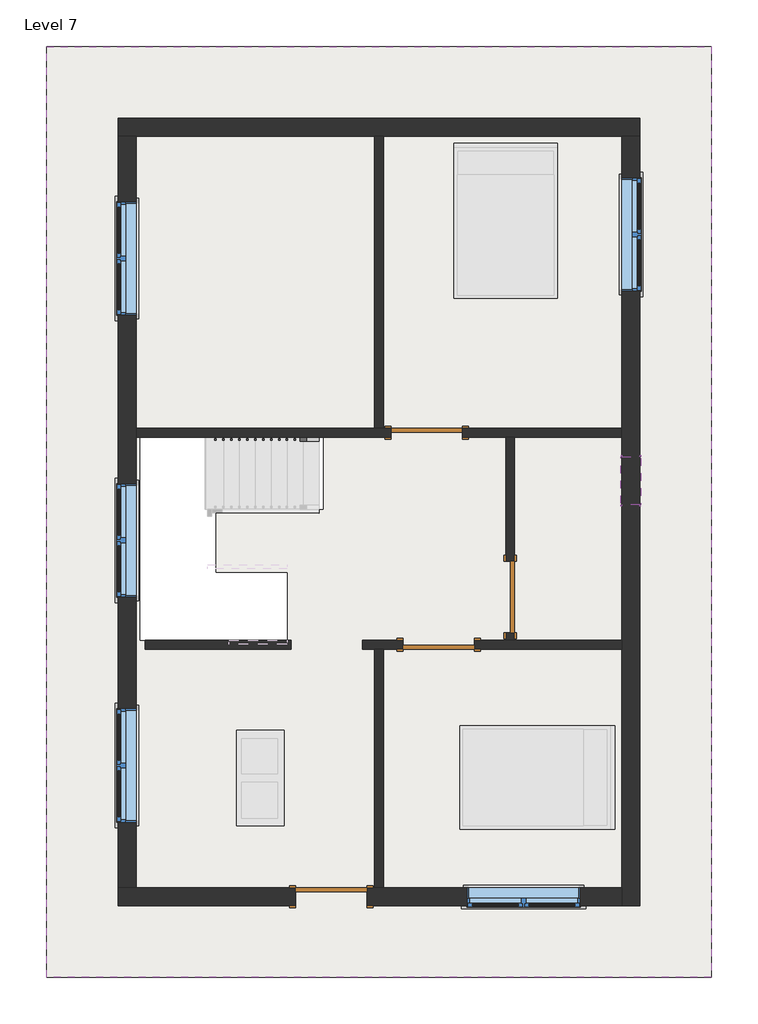
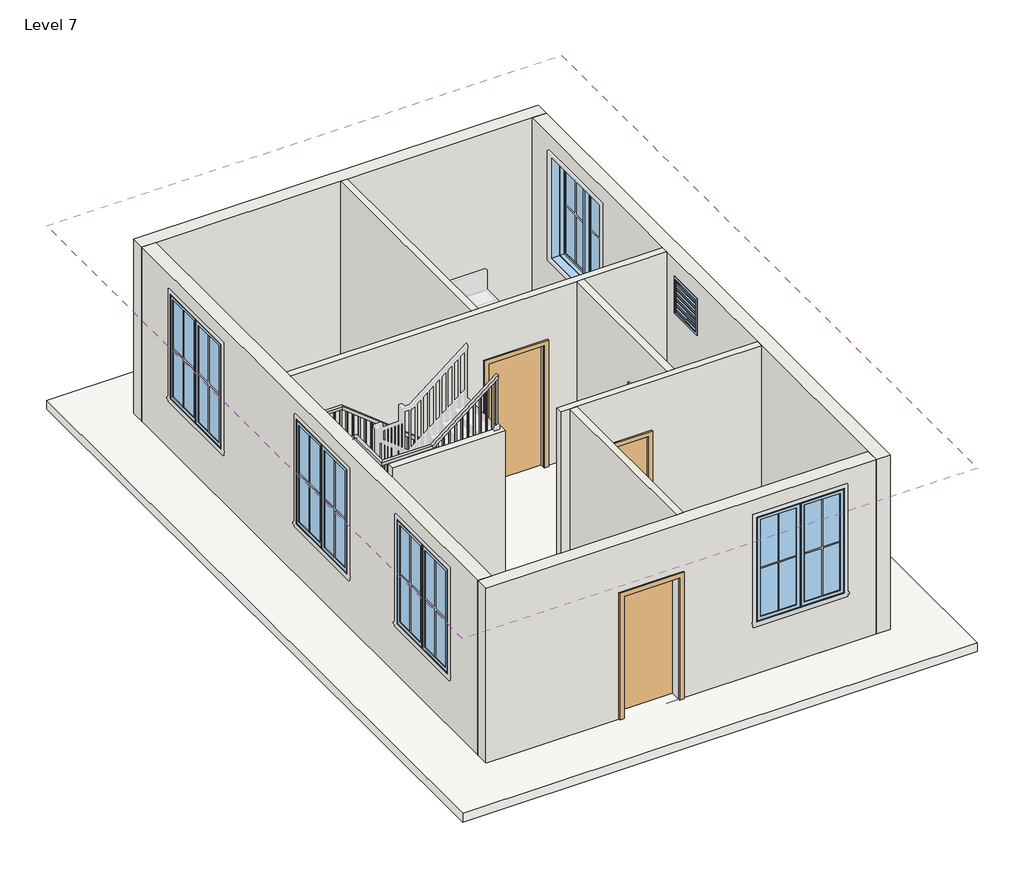
# One storey, part 1 of 2: 10 walls, 6 windows, 4 doors, 2 roofs, 1 railing, 1 slab.
"""IFC4 building model written with IfcOpenShell, lengths in millimetres."""

from ifc_helpers import new_model, si_unit, frame, origin, place, context, project, spatial, polyline, outline, extrude, faceted_brep, transform, mapped, element, save
from components import door_e5f9f3c4, door_0ca8825f, window_9ac97e1a, window_f2d8fef0

model = new_model("IFC4")

# Units and contexts
model_context = context("Model", 3, world=origin())
ifc_project = project(units=[si_unit("LENGTHUNIT", "METRE", prefix="MILLI")], contexts=[model_context])

# Site, building, storey
site = spatial("IfcSite", under=ifc_project)
building = spatial("IfcBuilding", under=site)
storey = spatial("IfcBuildingStorey", under=building, Name="Level 7", Elevation=16002.0)

# Doors
placement = place(None, origin())
door_shape = door_e5f9f3c4(model_context)
element("IfcDoor", 1, ObjectType="Single-Flush : 36\" x 84\"", at=placement, inside=storey, context=model_context, shape_type="MappedRepresentation", body=[
    mapped(door_shape, transform((-2225.1840247, 979.1819954, 16002.0), x_axis=(1.0, 0.0, 0.0), y_axis=(0.0, 1.0, 0.0), z_axis=(0.0, 0.0, 1.0))),
])
element("IfcDoor", 2, ObjectType="Single-Flush : 36\" x 84\"", at=placement, inside=storey, context=model_context, shape_type="MappedRepresentation", body=[
    mapped(door_shape, transform((-1158.3840247, -1116.3180046, 16002.0), x_axis=(0.0, -1.0, 0.0), y_axis=(1.0, 0.0, 0.0), z_axis=(0.0, 0.0, 1.0))),
])
element("IfcDoor", 3, ObjectType="Single-Flush : 36\" x 84\"", at=placement, inside=storey, context=model_context, shape_type="MappedRepresentation", body=[
    mapped(door_shape, transform((-2072.7840247, -1725.9180046, 16002.0), x_axis=(-1.0, 0.0, 0.0), y_axis=(0.0, -1.0, 0.0), z_axis=(0.0, 0.0, 1.0))),
])
door_2_shape = door_0ca8825f(model_context)
element("IfcDoor", 4, ObjectType="Single-Flush : 36\" x 84\"", at=placement, inside=storey, context=model_context, shape_type="MappedRepresentation", body=[
    mapped(door_2_shape, transform((-3444.3840247, -4945.3680046, 16002.0), x_axis=(1.0, 0.0, 0.0), y_axis=(0.0, 1.0, 0.0), z_axis=(0.0, 0.0, 1.0))),
])

# Railing
element("IfcRailing", 5, ObjectType="Handrail - Rectangular", at=placement, inside=storey, context=model_context, shape_type="SolidModel", body=[
    faceted_brep([(-3603.1340247, 871.2319954, 17076.8210526), (-3603.1340247, 871.2319954, 17012.0980109), (-3603.1340247, 922.0319954, 17012.0980109), (-3603.1340247, 922.0319954, 17076.8210526), (-5097.5006913, 871.2319954, 18256.5842105), (-5115.1365442, 871.2319954, 18205.7842105), (-5115.1365442, 922.0319954, 18205.7842105), (-5097.5006913, 922.0319954, 18256.5842105), (-5889.1340247, 871.2319954, 18256.5842105), (-5889.1340247, 871.2319954, 18205.7842105), (-5939.9340247, 922.0319954, 18205.7842105), (-5939.9340247, 922.0319954, 18256.5842105), (-5889.1340247, 130.6632454, 18256.5842105), (-5889.1340247, 112.1228815, 18205.7842105), (-5939.9340247, 112.1228815, 18205.7842105), (-5939.9340247, 130.6632454, 18256.5842105), (-5889.1340247, -877.3992546, 19105.4789474), (-5889.1340247, -895.9396185, 19054.6789474), (-5939.9340247, -895.9396185, 19054.6789474), (-5939.9340247, -877.3992546, 19105.4789474), (-5889.1340247, -1617.9680046, 19105.4789474), (-5889.1340247, -1617.9680046, 19054.6789474), (-5939.9340247, -1668.7680046, 19054.6789474), (-5939.9340247, -1668.7680046, 19105.4789474), (-5097.5006913, -1617.9680046, 19105.4789474), (-5079.8648385, -1617.9680046, 19054.6789474), (-5079.8648385, -1668.7680046, 19054.6789474), (-5097.5006913, -1668.7680046, 19105.4789474), (-4009.5340247, -1617.9680046, 19964.4), (-4009.5340247, -1668.7680046, 19964.4), (-4009.5340247, -1668.7680046, 19899.6769583), (-4009.5340247, -1617.9680046, 19899.6769583)], [[[0, 1, 2, 3]], [[1, 0, 4, 5]], [[2, 1, 5, 6]], [[3, 2, 6, 7]], [[0, 3, 7, 4]], [[5, 4, 8, 9]], [[6, 5, 9, 10]], [[7, 6, 10, 11]], [[4, 7, 11, 8]], [[9, 8, 12, 13]], [[10, 9, 13, 14]], [[11, 10, 14, 15]], [[8, 11, 15, 12]], [[13, 12, 16, 17]], [[14, 13, 17, 18]], [[15, 14, 18, 19]], [[12, 15, 19, 16]], [[17, 16, 20, 21]], [[18, 17, 21, 22]], [[19, 18, 22, 23]], [[16, 19, 23, 20]], [[21, 20, 24, 25]], [[22, 21, 25, 26]], [[23, 22, 26, 27]], [[20, 23, 27, 24]], [[28, 29, 30, 31]], [[25, 24, 28, 31]], [[26, 25, 31, 30]], [[27, 26, 30, 29]], [[24, 27, 29, 28]]]),
    extrude(outline(polyline([(19847.0388004, -4076.2090247), (19831.9993267, -4095.2590247), (18889.5789474, -4095.2590247), (18889.5789474, -4076.2090247), (19847.0388004, -4076.2090247)])), frame((0.0, -1652.8930046, 0.0), z_axis=(0.0, 1.0, 0.0), x_axis=(0.0, 0.0, 1.0)), (0.0, 0.0, 1.0), 19.05),
    extrude(outline(polyline([(19766.828274, -4177.8090247), (19751.7888004, -4196.8590247), (18889.5789474, -4196.8590247), (18889.5789474, -4177.8090247), (19766.828274, -4177.8090247)])), frame((0.0, -1652.8930046, 0.0), z_axis=(0.0, 1.0, 0.0), x_axis=(0.0, 0.0, 1.0)), (0.0, 0.0, 1.0), 19.05),
    extrude(outline(polyline([(19686.6177477, -4279.4090247), (19671.578274, -4298.4590247), (18729.1578947, -4298.4590247), (18729.1578947, -4279.4090247), (19686.6177477, -4279.4090247)])), frame((0.0, -1652.8930046, 0.0), z_axis=(0.0, 1.0, 0.0), x_axis=(0.0, 0.0, 1.0)), (0.0, 0.0, 1.0), 19.05),
    extrude(outline(polyline([(19606.4072214, -4381.0090247), (19591.3677477, -4400.0590247), (18729.1578947, -4400.0590247), (18729.1578947, -4381.0090247), (19606.4072214, -4381.0090247)])), frame((0.0, -1652.8930046, 0.0), z_axis=(0.0, 1.0, 0.0), x_axis=(0.0, 0.0, 1.0)), (0.0, 0.0, 1.0), 19.05),
    extrude(outline(polyline([(19526.1966951, -4482.6090247), (19511.1572214, -4501.6590247), (18568.7368421, -4501.6590247), (18568.7368421, -4482.6090247), (19526.1966951, -4482.6090247)])), frame((0.0, -1652.8930046, 0.0), z_axis=(0.0, 1.0, 0.0), x_axis=(0.0, 0.0, 1.0)), (0.0, 0.0, 1.0), 19.05),
    extrude(outline(polyline([(19445.9861688, -4584.2090247), (19430.9466951, -4603.2590247), (18568.7368421, -4603.2590247), (18568.7368421, -4584.2090247), (19445.9861688, -4584.2090247)])), frame((0.0, -1652.8930046, 0.0), z_axis=(0.0, 1.0, 0.0), x_axis=(0.0, 0.0, 1.0)), (0.0, 0.0, 1.0), 19.05),
    extrude(outline(polyline([(19365.7756425, -4685.8090247), (19350.7361688, -4704.8590247), (18408.3157895, -4704.8590247), (18408.3157895, -4685.8090247), (19365.7756425, -4685.8090247)])), frame((0.0, -1652.8930046, 0.0), z_axis=(0.0, 1.0, 0.0), x_axis=(0.0, 0.0, 1.0)), (0.0, 0.0, 1.0), 19.05),
    extrude(outline(polyline([(19285.5651161, -4787.4090247), (19270.5256425, -4806.4590247), (18408.3157895, -4806.4590247), (18408.3157895, -4787.4090247), (19285.5651161, -4787.4090247)])), frame((0.0, -1652.8930046, 0.0), z_axis=(0.0, 1.0, 0.0), x_axis=(0.0, 0.0, 1.0)), (0.0, 0.0, 1.0), 19.05),
    extrude(outline(polyline([(19205.3545898, -4889.0090247), (19190.3151161, -4908.0590247), (18247.8947368, -4908.0590247), (18247.8947368, -4889.0090247), (19205.3545898, -4889.0090247)])), frame((0.0, -1652.8930046, 0.0), z_axis=(0.0, 1.0, 0.0), x_axis=(0.0, 0.0, 1.0)), (0.0, 0.0, 1.0), 19.05),
    extrude(outline(polyline([(19125.1440635, -4990.6090247), (19110.1045898, -5009.6590247), (18247.8947368, -5009.6590247), (18247.8947368, -4990.6090247), (19125.1440635, -4990.6090247)])), frame((0.0, -1652.8930046, 0.0), z_axis=(0.0, 1.0, 0.0), x_axis=(0.0, 0.0, 1.0)), (0.0, 0.0, 1.0), 19.05),
    extrude(outline(polyline([(-5111.2590247, -1652.8930046), (-5111.2590247, -1633.8430046), (-5092.2090247, -1633.8430046), (-5092.2090247, -1652.8930046), (-5111.2590247, -1652.8930046)])), frame((0.0, 0.0, 18087.4736842), z_axis=(0.0, 0.0, 1.0), x_axis=(1.0, 0.0, 0.0)), (0.0, 0.0, 1.0), 967.2052632),
    extrude(outline(polyline([(-5212.8590247, -1652.8930046), (-5212.8590247, -1633.8430046), (-5193.8090247, -1633.8430046), (-5193.8090247, -1652.8930046), (-5212.8590247, -1652.8930046)])), frame((0.0, 0.0, 18087.4736842), z_axis=(0.0, 0.0, 1.0), x_axis=(1.0, 0.0, 0.0)), (0.0, 0.0, 1.0), 967.2052632),
    extrude(outline(polyline([(-5314.4590247, -1652.8930046), (-5314.4590247, -1633.8430046), (-5295.4090247, -1633.8430046), (-5295.4090247, -1652.8930046), (-5314.4590247, -1652.8930046)])), frame((0.0, 0.0, 18087.4736842), z_axis=(0.0, 0.0, 1.0), x_axis=(1.0, 0.0, 0.0)), (0.0, 0.0, 1.0), 967.2052632),
    extrude(outline(polyline([(-5416.0590247, -1652.8930046), (-5416.0590247, -1633.8430046), (-5397.0090247, -1633.8430046), (-5397.0090247, -1652.8930046), (-5416.0590247, -1652.8930046)])), frame((0.0, 0.0, 18087.4736842), z_axis=(0.0, 0.0, 1.0), x_axis=(1.0, 0.0, 0.0)), (0.0, 0.0, 1.0), 967.2052632),
    extrude(outline(polyline([(-5517.6590247, -1652.8930046), (-5517.6590247, -1633.8430046), (-5498.6090247, -1633.8430046), (-5498.6090247, -1652.8930046), (-5517.6590247, -1652.8930046)])), frame((0.0, 0.0, 18087.4736842), z_axis=(0.0, 0.0, 1.0), x_axis=(1.0, 0.0, 0.0)), (0.0, 0.0, 1.0), 967.2052632),
    extrude(outline(polyline([(-5619.2590247, -1652.8930046), (-5619.2590247, -1633.8430046), (-5600.2090247, -1633.8430046), (-5600.2090247, -1652.8930046), (-5619.2590247, -1652.8930046)])), frame((0.0, 0.0, 18087.4736842), z_axis=(0.0, 0.0, 1.0), x_axis=(1.0, 0.0, 0.0)), (0.0, 0.0, 1.0), 967.2052632),
    extrude(outline(polyline([(-5720.8590247, -1652.8930046), (-5720.8590247, -1633.8430046), (-5701.8090247, -1633.8430046), (-5701.8090247, -1652.8930046), (-5720.8590247, -1652.8930046)])), frame((0.0, 0.0, 18087.4736842), z_axis=(0.0, 0.0, 1.0), x_axis=(1.0, 0.0, 0.0)), (0.0, 0.0, 1.0), 967.2052632),
    extrude(outline(polyline([(-5822.4590247, -1652.8930046), (-5822.4590247, -1633.8430046), (-5803.4090247, -1633.8430046), (-5803.4090247, -1652.8930046), (-5822.4590247, -1652.8930046)])), frame((0.0, 0.0, 18087.4736842), z_axis=(0.0, 0.0, 1.0), x_axis=(1.0, 0.0, 0.0)), (0.0, 0.0, 1.0), 967.2052632),
    extrude(outline(polyline([(-5924.0590247, -1532.2430046), (-5905.0090247, -1532.2430046), (-5905.0090247, -1551.2930046), (-5924.0590247, -1551.2930046), (-5924.0590247, -1532.2430046)])), frame((0.0, 0.0, 18087.4736842), z_axis=(0.0, 0.0, 1.0), x_axis=(1.0, 0.0, 0.0)), (0.0, 0.0, 1.0), 967.2052632),
    extrude(outline(polyline([(-5924.0590247, -1430.6430046), (-5905.0090247, -1430.6430046), (-5905.0090247, -1449.6930046), (-5924.0590247, -1449.6930046), (-5924.0590247, -1430.6430046)])), frame((0.0, 0.0, 18087.4736842), z_axis=(0.0, 0.0, 1.0), x_axis=(1.0, 0.0, 0.0)), (0.0, 0.0, 1.0), 967.2052632),
    extrude(outline(polyline([(-5924.0590247, -1329.0430046), (-5905.0090247, -1329.0430046), (-5905.0090247, -1348.0930046), (-5924.0590247, -1348.0930046), (-5924.0590247, -1329.0430046)])), frame((0.0, 0.0, 18087.4736842), z_axis=(0.0, 0.0, 1.0), x_axis=(1.0, 0.0, 0.0)), (0.0, 0.0, 1.0), 967.2052632),
    extrude(outline(polyline([(-5924.0590247, -1227.4430046), (-5905.0090247, -1227.4430046), (-5905.0090247, -1246.4930046), (-5924.0590247, -1246.4930046), (-5924.0590247, -1227.4430046)])), frame((0.0, 0.0, 18087.4736842), z_axis=(0.0, 0.0, 1.0), x_axis=(1.0, 0.0, 0.0)), (0.0, 0.0, 1.0), 967.2052632),
    extrude(outline(polyline([(-5924.0590247, -1125.8430046), (-5905.0090247, -1125.8430046), (-5905.0090247, -1144.8930046), (-5924.0590247, -1144.8930046), (-5924.0590247, -1125.8430046)])), frame((0.0, 0.0, 18087.4736842), z_axis=(0.0, 0.0, 1.0), x_axis=(1.0, 0.0, 0.0)), (0.0, 0.0, 1.0), 967.2052632),
    extrude(outline(polyline([(-5924.0590247, -1024.2430046), (-5905.0090247, -1024.2430046), (-5905.0090247, -1043.2930046), (-5924.0590247, -1043.2930046), (-5924.0590247, -1024.2430046)])), frame((0.0, 0.0, 18087.4736842), z_axis=(0.0, 0.0, 1.0), x_axis=(1.0, 0.0, 0.0)), (0.0, 0.0, 1.0), 967.2052632),
    extrude(outline(polyline([(-5924.0590247, -922.6430046), (-5905.0090247, -922.6430046), (-5905.0090247, -941.6930046), (-5924.0590247, -941.6930046), (-5924.0590247, -922.6430046)])), frame((0.0, 0.0, 18087.4736842), z_axis=(0.0, 0.0, 1.0), x_axis=(1.0, 0.0, 0.0)), (0.0, 0.0, 1.0), 967.2052632),
    extrude(outline(polyline([(-840.0930046, 19007.6502199), (-821.0430046, 18991.6081146), (-821.0430046, 18087.4736842), (-840.0930046, 18087.4736842), (-840.0930046, 19007.6502199)])), frame((-5924.0590247, 0.0, 0.0), z_axis=(1.0, 0.0, 0.0), x_axis=(0.0, 1.0, 0.0)), (0.0, 0.0, 1.0), 19.05),
    extrude(outline(polyline([(-738.4930046, 18922.0923251), (-719.4430046, 18906.0502199), (-719.4430046, 17927.0526316), (-738.4930046, 17927.0526316), (-738.4930046, 18922.0923251)])), frame((-5924.0590247, 0.0, 0.0), z_axis=(1.0, 0.0, 0.0), x_axis=(0.0, 1.0, 0.0)), (0.0, 0.0, 1.0), 19.05),
    extrude(outline(polyline([(-636.8930046, 18836.5344304), (-617.8430046, 18820.4923251), (-617.8430046, 17927.0526316), (-636.8930046, 17927.0526316), (-636.8930046, 18836.5344304)])), frame((-5924.0590247, 0.0, 0.0), z_axis=(1.0, 0.0, 0.0), x_axis=(0.0, 1.0, 0.0)), (0.0, 0.0, 1.0), 19.05),
    extrude(outline(polyline([(-535.2930046, 18750.9765357), (-516.2430046, 18734.9344304), (-516.2430046, 17766.6315789), (-535.2930046, 17766.6315789), (-535.2930046, 18750.9765357)])), frame((-5924.0590247, 0.0, 0.0), z_axis=(1.0, 0.0, 0.0), x_axis=(0.0, 1.0, 0.0)), (0.0, 0.0, 1.0), 19.05),
    extrude(outline(polyline([(-433.6930046, 18665.4186409), (-414.6430046, 18649.3765357), (-414.6430046, 17766.6315789), (-433.6930046, 17766.6315789), (-433.6930046, 18665.4186409)])), frame((-5924.0590247, 0.0, 0.0), z_axis=(1.0, 0.0, 0.0), x_axis=(0.0, 1.0, 0.0)), (0.0, 0.0, 1.0), 19.05),
    extrude(outline(polyline([(-332.0930046, 18579.8607462), (-313.0430046, 18563.8186409), (-313.0430046, 17606.2105263), (-332.0930046, 17606.2105263), (-332.0930046, 18579.8607462)])), frame((-5924.0590247, 0.0, 0.0), z_axis=(1.0, 0.0, 0.0), x_axis=(0.0, 1.0, 0.0)), (0.0, 0.0, 1.0), 19.05),
    extrude(outline(polyline([(-230.4930046, 18494.3028514), (-211.4430046, 18478.2607462), (-211.4430046, 17606.2105263), (-230.4930046, 17606.2105263), (-230.4930046, 18494.3028514)])), frame((-5924.0590247, 0.0, 0.0), z_axis=(1.0, 0.0, 0.0), x_axis=(0.0, 1.0, 0.0)), (0.0, 0.0, 1.0), 19.05),
    extrude(outline(polyline([(-128.8930046, 18408.7449567), (-109.8430046, 18392.7028514), (-109.8430046, 17445.7894737), (-128.8930046, 17445.7894737), (-128.8930046, 18408.7449567)])), frame((-5924.0590247, 0.0, 0.0), z_axis=(1.0, 0.0, 0.0), x_axis=(0.0, 1.0, 0.0)), (0.0, 0.0, 1.0), 19.05),
    extrude(outline(polyline([(-27.2930046, 18323.187062), (-8.2430046, 18307.1449567), (-8.2430046, 17445.7894737), (-27.2930046, 17445.7894737), (-27.2930046, 18323.187062)])), frame((-5924.0590247, 0.0, 0.0), z_axis=(1.0, 0.0, 0.0), x_axis=(0.0, 1.0, 0.0)), (0.0, 0.0, 1.0), 19.05),
    extrude(outline(polyline([(74.3069954, 18237.6291672), (93.3569954, 18221.587062), (93.3569954, 17285.3684211), (74.3069954, 17285.3684211), (74.3069954, 18237.6291672)])), frame((-5924.0590247, 0.0, 0.0), z_axis=(1.0, 0.0, 0.0), x_axis=(0.0, 1.0, 0.0)), (0.0, 0.0, 1.0), 19.05),
    extrude(outline(polyline([(-5924.0590247, 194.9569954), (-5905.0090247, 194.9569954), (-5905.0090247, 175.9069954), (-5924.0590247, 175.9069954), (-5924.0590247, 194.9569954)])), frame((0.0, 0.0, 17285.3684211), z_axis=(0.0, 0.0, 1.0), x_axis=(1.0, 0.0, 0.0)), (0.0, 0.0, 1.0), 920.4157895),
    extrude(outline(polyline([(-5924.0590247, 296.5569954), (-5905.0090247, 296.5569954), (-5905.0090247, 277.5069954), (-5924.0590247, 277.5069954), (-5924.0590247, 296.5569954)])), frame((0.0, 0.0, 17285.3684211), z_axis=(0.0, 0.0, 1.0), x_axis=(1.0, 0.0, 0.0)), (0.0, 0.0, 1.0), 920.4157895),
    extrude(outline(polyline([(-5924.0590247, 398.1569954), (-5905.0090247, 398.1569954), (-5905.0090247, 379.1069954), (-5924.0590247, 379.1069954), (-5924.0590247, 398.1569954)])), frame((0.0, 0.0, 17285.3684211), z_axis=(0.0, 0.0, 1.0), x_axis=(1.0, 0.0, 0.0)), (0.0, 0.0, 1.0), 920.4157895),
    extrude(outline(polyline([(-5924.0590247, 499.7569954), (-5905.0090247, 499.7569954), (-5905.0090247, 480.7069954), (-5924.0590247, 480.7069954), (-5924.0590247, 499.7569954)])), frame((0.0, 0.0, 17285.3684211), z_axis=(0.0, 0.0, 1.0), x_axis=(1.0, 0.0, 0.0)), (0.0, 0.0, 1.0), 920.4157895),
    extrude(outline(polyline([(-5924.0590247, 601.3569954), (-5905.0090247, 601.3569954), (-5905.0090247, 582.3069954), (-5924.0590247, 582.3069954), (-5924.0590247, 601.3569954)])), frame((0.0, 0.0, 17285.3684211), z_axis=(0.0, 0.0, 1.0), x_axis=(1.0, 0.0, 0.0)), (0.0, 0.0, 1.0), 920.4157895),
    extrude(outline(polyline([(-5924.0590247, 702.9569954), (-5905.0090247, 702.9569954), (-5905.0090247, 683.9069954), (-5924.0590247, 683.9069954), (-5924.0590247, 702.9569954)])), frame((0.0, 0.0, 17285.3684211), z_axis=(0.0, 0.0, 1.0), x_axis=(1.0, 0.0, 0.0)), (0.0, 0.0, 1.0), 920.4157895),
    extrude(outline(polyline([(-5924.0590247, 804.5569954), (-5905.0090247, 804.5569954), (-5905.0090247, 785.5069954), (-5924.0590247, 785.5069954), (-5924.0590247, 804.5569954)])), frame((0.0, 0.0, 17285.3684211), z_axis=(0.0, 0.0, 1.0), x_axis=(1.0, 0.0, 0.0)), (0.0, 0.0, 1.0), 920.4157895),
    extrude(outline(polyline([(-5828.8090247, 906.1569954), (-5828.8090247, 887.1069954), (-5847.8590247, 887.1069954), (-5847.8590247, 906.1569954), (-5828.8090247, 906.1569954)])), frame((0.0, 0.0, 17285.3684211), z_axis=(0.0, 0.0, 1.0), x_axis=(1.0, 0.0, 0.0)), (0.0, 0.0, 1.0), 920.4157895),
    extrude(outline(polyline([(-5727.2090247, 906.1569954), (-5727.2090247, 887.1069954), (-5746.2590247, 887.1069954), (-5746.2590247, 906.1569954), (-5727.2090247, 906.1569954)])), frame((0.0, 0.0, 17285.3684211), z_axis=(0.0, 0.0, 1.0), x_axis=(1.0, 0.0, 0.0)), (0.0, 0.0, 1.0), 920.4157895),
    extrude(outline(polyline([(-5625.6090247, 906.1569954), (-5625.6090247, 887.1069954), (-5644.6590247, 887.1069954), (-5644.6590247, 906.1569954), (-5625.6090247, 906.1569954)])), frame((0.0, 0.0, 17285.3684211), z_axis=(0.0, 0.0, 1.0), x_axis=(1.0, 0.0, 0.0)), (0.0, 0.0, 1.0), 920.4157895),
    extrude(outline(polyline([(-5524.0090247, 906.1569954), (-5524.0090247, 887.1069954), (-5543.0590247, 887.1069954), (-5543.0590247, 906.1569954), (-5524.0090247, 906.1569954)])), frame((0.0, 0.0, 17285.3684211), z_axis=(0.0, 0.0, 1.0), x_axis=(1.0, 0.0, 0.0)), (0.0, 0.0, 1.0), 920.4157895),
    extrude(outline(polyline([(-5422.4090247, 906.1569954), (-5422.4090247, 887.1069954), (-5441.4590247, 887.1069954), (-5441.4590247, 906.1569954), (-5422.4090247, 906.1569954)])), frame((0.0, 0.0, 17285.3684211), z_axis=(0.0, 0.0, 1.0), x_axis=(1.0, 0.0, 0.0)), (0.0, 0.0, 1.0), 920.4157895),
    extrude(outline(polyline([(-5320.8090247, 906.1569954), (-5320.8090247, 887.1069954), (-5339.8590247, 887.1069954), (-5339.8590247, 906.1569954), (-5320.8090247, 906.1569954)])), frame((0.0, 0.0, 17285.3684211), z_axis=(0.0, 0.0, 1.0), x_axis=(1.0, 0.0, 0.0)), (0.0, 0.0, 1.0), 920.4157895),
    extrude(outline(polyline([(-5219.2090247, 906.1569954), (-5219.2090247, 887.1069954), (-5238.2590247, 887.1069954), (-5238.2590247, 906.1569954), (-5219.2090247, 906.1569954)])), frame((0.0, 0.0, 17285.3684211), z_axis=(0.0, 0.0, 1.0), x_axis=(1.0, 0.0, 0.0)), (0.0, 0.0, 1.0), 920.4157895),
    extrude(outline(polyline([(-5117.6090247, 906.1569954), (-5117.6090247, 887.1069954), (-5136.6590247, 887.1069954), (-5136.6590247, 906.1569954), (-5117.6090247, 906.1569954)])), frame((0.0, 0.0, 17285.3684211), z_axis=(0.0, 0.0, 1.0), x_axis=(1.0, 0.0, 0.0)), (0.0, 0.0, 1.0), 920.4157895),
    extrude(outline(polyline([(18127.5256425, -5016.0090247), (18142.5651161, -5035.0590247), (17285.3684211, -5035.0590247), (17285.3684211, -5016.0090247), (18127.5256425, -5016.0090247)])), frame((0.0, 887.1069954, 0.0), z_axis=(0.0, 1.0, 0.0), x_axis=(0.0, 0.0, 1.0)), (0.0, 0.0, 1.0), 19.05),
    extrude(outline(polyline([(18047.3151161, -4914.4090247), (18062.3545898, -4933.4590247), (17124.9473684, -4933.4590247), (17124.9473684, -4914.4090247), (18047.3151161, -4914.4090247)])), frame((0.0, 887.1069954, 0.0), z_axis=(0.0, 1.0, 0.0), x_axis=(0.0, 0.0, 1.0)), (0.0, 0.0, 1.0), 19.05),
    extrude(outline(polyline([(17967.1045898, -4812.8090247), (17982.1440635, -4831.8590247), (17124.9473684, -4831.8590247), (17124.9473684, -4812.8090247), (17967.1045898, -4812.8090247)])), frame((0.0, 887.1069954, 0.0), z_axis=(0.0, 1.0, 0.0), x_axis=(0.0, 0.0, 1.0)), (0.0, 0.0, 1.0), 19.05),
    extrude(outline(polyline([(17886.8940635, -4711.2090247), (17901.9335372, -4730.2590247), (16964.5263158, -4730.2590247), (16964.5263158, -4711.2090247), (17886.8940635, -4711.2090247)])), frame((0.0, 887.1069954, 0.0), z_axis=(0.0, 1.0, 0.0), x_axis=(0.0, 0.0, 1.0)), (0.0, 0.0, 1.0), 19.05),
    extrude(outline(polyline([(17806.6835372, -4609.6090247), (17821.7230109, -4628.6590247), (16964.5263158, -4628.6590247), (16964.5263158, -4609.6090247), (17806.6835372, -4609.6090247)])), frame((0.0, 887.1069954, 0.0), z_axis=(0.0, 1.0, 0.0), x_axis=(0.0, 0.0, 1.0)), (0.0, 0.0, 1.0), 19.05),
    extrude(outline(polyline([(17726.4730109, -4508.0090247), (17741.5124846, -4527.0590247), (16804.1052632, -4527.0590247), (16804.1052632, -4508.0090247), (17726.4730109, -4508.0090247)])), frame((0.0, 887.1069954, 0.0), z_axis=(0.0, 1.0, 0.0), x_axis=(0.0, 0.0, 1.0)), (0.0, 0.0, 1.0), 19.05),
    extrude(outline(polyline([(17646.2624846, -4406.4090247), (17661.3019583, -4425.4590247), (16804.1052632, -4425.4590247), (16804.1052632, -4406.4090247), (17646.2624846, -4406.4090247)])), frame((0.0, 887.1069954, 0.0), z_axis=(0.0, 1.0, 0.0), x_axis=(0.0, 0.0, 1.0)), (0.0, 0.0, 1.0), 19.05),
    extrude(outline(polyline([(17566.0519583, -4304.8090247), (17581.0914319, -4323.8590247), (16643.6842105, -4323.8590247), (16643.6842105, -4304.8090247), (17566.0519583, -4304.8090247)])), frame((0.0, 887.1069954, 0.0), z_axis=(0.0, 1.0, 0.0), x_axis=(0.0, 0.0, 1.0)), (0.0, 0.0, 1.0), 19.05),
    extrude(outline(polyline([(17485.8414319, -4203.2090247), (17500.8809056, -4222.2590247), (16643.6842105, -4222.2590247), (16643.6842105, -4203.2090247), (17485.8414319, -4203.2090247)])), frame((0.0, 887.1069954, 0.0), z_axis=(0.0, 1.0, 0.0), x_axis=(0.0, 0.0, 1.0)), (0.0, 0.0, 1.0), 19.05),
    extrude(outline(polyline([(17405.6309056, -4101.6090247), (17420.6703793, -4120.6590247), (16483.2631579, -4120.6590247), (16483.2631579, -4101.6090247), (17405.6309056, -4101.6090247)])), frame((0.0, 887.1069954, 0.0), z_axis=(0.0, 1.0, 0.0), x_axis=(0.0, 0.0, 1.0)), (0.0, 0.0, 1.0), 19.05),
    extrude(outline(polyline([(17325.4203793, -4000.0090247), (17340.459853, -4019.0590247), (16483.2631579, -4019.0590247), (16483.2631579, -4000.0090247), (17325.4203793, -4000.0090247)])), frame((0.0, 887.1069954, 0.0), z_axis=(0.0, 1.0, 0.0), x_axis=(0.0, 0.0, 1.0)), (0.0, 0.0, 1.0), 19.05),
    extrude(outline(polyline([(17245.209853, -3898.4090247), (17260.2493267, -3917.4590247), (16322.8421053, -3917.4590247), (16322.8421053, -3898.4090247), (17245.209853, -3898.4090247)])), frame((0.0, 887.1069954, 0.0), z_axis=(0.0, 1.0, 0.0), x_axis=(0.0, 0.0, 1.0)), (0.0, 0.0, 1.0), 19.05),
    extrude(outline(polyline([(17164.9993267, -3796.8090247), (17180.0388004, -3815.8590247), (16322.8421053, -3815.8590247), (16322.8421053, -3796.8090247), (17164.9993267, -3796.8090247)])), frame((0.0, 887.1069954, 0.0), z_axis=(0.0, 1.0, 0.0), x_axis=(0.0, 0.0, 1.0)), (0.0, 0.0, 1.0), 19.05),
    extrude(outline(polyline([(17084.7888004, -3695.2090247), (17099.828274, -3714.2590247), (16162.4210526, -3714.2590247), (16162.4210526, -3695.2090247), (17084.7888004, -3695.2090247)])), frame((0.0, 887.1069954, 0.0), z_axis=(0.0, 1.0, 0.0), x_axis=(0.0, 0.0, 1.0)), (0.0, 0.0, 1.0), 19.05),
    extrude(outline(polyline([(-5924.0590247, -1633.8430046), (-5905.0090247, -1633.8430046), (-5905.0090247, -1652.8930046), (-5924.0590247, -1652.8930046), (-5924.0590247, -1633.8430046)])), frame((0.0, 0.0, 18087.4736842), z_axis=(0.0, 0.0, 1.0), x_axis=(1.0, 0.0, 0.0)), (0.0, 0.0, 1.0), 967.2052632),
    extrude(outline(polyline([(-5905.0090247, 906.1569954), (-5905.0090247, 887.1069954), (-5924.0590247, 887.1069954), (-5924.0590247, 906.1569954), (-5905.0090247, 906.1569954)])), frame((0.0, 0.0, 17285.3684211), z_axis=(0.0, 0.0, 1.0), x_axis=(1.0, 0.0, 0.0)), (0.0, 0.0, 1.0), 920.4157895),
    extrude(outline(polyline([(19899.6769583, -4009.5340247), (19884.6374846, -4028.5840247), (18889.5789474, -4028.5840247), (18889.5789474, -4009.5340247), (19899.6769583, -4009.5340247)])), frame((0.0, -1652.8930046, 0.0), z_axis=(0.0, 1.0, 0.0), x_axis=(0.0, 0.0, 1.0)), (0.0, 0.0, 1.0), 19.05),
    extrude(outline(polyline([(17012.0980109, -3603.1340247), (17027.1374846, -3622.1840247), (16162.4210526, -3622.1840247), (16162.4210526, -3603.1340247), (17012.0980109, -3603.1340247)])), frame((0.0, 887.1069954, 0.0), z_axis=(0.0, 1.0, 0.0), x_axis=(0.0, 0.0, 1.0)), (0.0, 0.0, 1.0), 19.05),
])

# Roofs
element("IfcRoof", 6, ObjectType="ROOF 6\"", at=placement, inside=storey, context=model_context, shape_type="SweptSolid", body=[
    extrude(outline(polyline([(-7082.9340247, 5913.1319954), (1413.3659753, 5913.1319954), (1413.3659753, -5974.0680046), (-7082.9340247, -5974.0680046), (-7082.9340247, 5913.1319954)]), holes=[polyline([(-5889.1340247, 922.0319954), (-5889.1340247, -1668.7680046), (-4009.5340247, -1668.7680046), (-4009.5340247, -805.1680046), (-4923.9340247, -805.1680046), (-4923.9340247, 7.6319954), (-3552.3340247, 7.6319954), (-3552.3340247, 922.0319954), (-5889.1340247, 922.0319954)])]), frame((0.0, 0.0, 15849.6), z_axis=(0.0, 0.0, 1.0), x_axis=(1.0, 0.0, 0.0)), (0.0, 0.0, 1.0), 152.4),
])
element("IfcRoof", 7, ObjectType="ROOF 6\"", at=placement, inside=storey, context=model_context, shape_type="SweptSolid", body=[
    extrude(outline(polyline([(-7082.9340247, 5913.1319954), (1413.3659753, 5913.1319954), (1413.3659753, -5974.0680046), (-7082.9340247, -5974.0680046), (-7082.9340247, 5913.1319954)]), holes=[polyline([(-5889.1340247, 922.0319954), (-5889.1340247, -1668.7680046), (-4009.5340247, -1668.7680046), (-4009.5340247, -805.1680046), (-4923.9340247, -805.1680046), (-4923.9340247, 7.6319954), (-3552.3340247, 7.6319954), (-3552.3340247, 922.0319954), (-5889.1340247, 922.0319954)])]), frame((0.0, 0.0, 19050.0), z_axis=(0.0, 0.0, 1.0), x_axis=(1.0, 0.0, 0.0)), (0.0, 0.0, 1.0), 152.4),
])

# Slab
element("IfcSlab", 8, ObjectType="FLOOR 6\"", at=placement, inside=storey, context=model_context, shape_type="SweptSolid", body=[
    extrude(outline(polyline([(498.9659753, 4998.7319954), (498.9659753, -5059.6680046), (-6168.5340247, -5059.6680046), (-6168.5340247, 4998.7319954), (498.9659753, 4998.7319954)]), holes=[polyline([(-5889.1340247, 922.0319954), (-5889.1340247, -1668.7680046), (-4009.5340247, -1668.7680046), (-4009.5340247, -805.1680046), (-4923.9340247, -805.1680046), (-4923.9340247, 7.6319954), (-3552.3340247, 7.6319954), (-3552.3340247, 922.0319954), (-5889.1340247, 922.0319954)])]), frame((0.0, 0.0, 15849.6), z_axis=(0.0, 0.0, 1.0), x_axis=(1.0, 0.0, 0.0)), (0.0, 0.0, 1.0), 152.4),
])

# Walls
element("IfcWall", 9, ObjectType="WALL 4.5\"", at=placement, inside=storey, context=model_context, shape_type="SweptSolid", body=[
    extrude(outline(polyline([(-2891.9340247, 1036.3319954), (-2891.9340247, 4770.1319954), (-2777.6340247, 4770.1319954), (-2777.6340247, 1036.3319954), (-2891.9340247, 1036.3319954)])), frame((0.0, 0.0, 16002.0), z_axis=(0.0, 0.0, 1.0), x_axis=(1.0, 0.0, 0.0)), (0.0, 0.0, 1.0), 3048.0),
])
element("IfcWall", 10, ObjectType="WALL 4.5\"", at=placement, inside=storey, context=model_context, shape_type="Brep", body=[
    faceted_brep([(-1767.9840247, 922.0319954, 18135.6), (-1767.9840247, 922.0319954, 16002.0), (-1215.5340247, 922.0319954, 16002.0), (-1101.2340247, 922.0319954, 16002.0), (270.3659753, 922.0319954, 16002.0), (270.3659753, 922.0319954, 19050.0), (-1101.2340247, 922.0319954, 19050.0), (-1215.5340247, 922.0319954, 19050.0), (-3552.3340247, 922.0319954, 19050.0), (-5889.1340247, 922.0319954, 19050.0), (-5939.9340247, 922.0319954, 19050.0), (-5939.9340247, 922.0319954, 16002.0), (-2682.3840247, 922.0319954, 16002.0), (-2682.3840247, 922.0319954, 18135.6), (270.3659753, 1036.3319954, 16002.0), (-1767.9840247, 1036.3319954, 16002.0), (-1767.9840247, 1036.3319954, 18135.6), (-2682.3840247, 1036.3319954, 18135.6), (-2682.3840247, 1036.3319954, 16002.0), (-2777.6340247, 1036.3319954, 16002.0), (-2891.9340247, 1036.3319954, 16002.0), (-5939.9340247, 1036.3319954, 16002.0), (-5939.9340247, 1036.3319954, 19050.0), (-2891.9340247, 1036.3319954, 19050.0), (-2777.6340247, 1036.3319954, 19050.0), (270.3659753, 1036.3319954, 19050.0)], [[[0, 1, 2, 3, 4, 5, 6, 7, 8, 9, 10, 11, 12, 13]], [[14, 15, 16, 17, 18, 19, 20, 21, 22, 23, 24, 25]], [[12, 11, 21, 20, 19, 18]], [[4, 3, 2, 1, 15, 14]], [[5, 4, 14, 25]], [[11, 10, 22, 21]], [[16, 15, 1, 0]], [[17, 16, 0, 13]], [[18, 17, 13, 12]], [[10, 9, 8, 7, 6, 5, 25, 24, 23, 22]]]),
])
element("IfcWall", 11, ObjectType="WALL 4.5\"", at=placement, inside=storey, context=model_context, shape_type="SweptSolid", body=[
    extrude(outline(polyline([(-1573.5180046, 18135.6), (-1573.5180046, 16002.0), (-1668.7680046, 16002.0), (-1668.7680046, 19050.0), (922.0319954, 19050.0), (922.0319954, 16002.0), (-659.1180046, 16002.0), (-659.1180046, 18135.6), (-1573.5180046, 18135.6)])), frame((-1215.5340247, 0.0, 0.0), z_axis=(1.0, 0.0, 0.0), x_axis=(0.0, 1.0, 0.0)), (0.0, 0.0, 1.0), 114.3),
])
element("IfcWall", 12, ObjectType="WALL 4.5\"", at=placement, inside=storey, context=model_context, shape_type="Brep", body=[
    faceted_brep([(-2529.9840247, -1668.7680046, 18135.6), (-2529.9840247, -1668.7680046, 16002.0), (-3044.3340247, -1668.7680046, 16002.0), (-3044.3340247, -1668.7680046, 19050.0), (-1215.5340247, -1668.7680046, 19050.0), (-1101.2340247, -1668.7680046, 19050.0), (270.3659753, -1668.7680046, 19050.0), (270.3659753, -1668.7680046, 16002.0), (-1101.2340247, -1668.7680046, 16002.0), (-1215.5340247, -1668.7680046, 16002.0), (-1615.5840247, -1668.7680046, 16002.0), (-1615.5840247, -1668.7680046, 18135.6), (-3044.3340247, -1783.0680046, 16002.0), (-2891.9340247, -1783.0680046, 16002.0), (-2777.6340247, -1783.0680046, 16002.0), (-2529.9840247, -1783.0680046, 16002.0), (-2529.9840247, -1783.0680046, 18135.6), (-1615.5840247, -1783.0680046, 18135.6), (-1615.5840247, -1783.0680046, 16002.0), (270.3659753, -1783.0680046, 16002.0), (270.3659753, -1783.0680046, 19050.0), (-2777.6340247, -1783.0680046, 19050.0), (-2891.9340247, -1783.0680046, 19050.0), (-3044.3340247, -1783.0680046, 19050.0)], [[[0, 1, 2, 3, 4, 5, 6, 7, 8, 9, 10, 11]], [[12, 13, 14, 15, 16, 17, 18, 19, 20, 21, 22, 23]], [[2, 1, 15, 14, 13, 12]], [[10, 9, 8, 7, 19, 18]], [[3, 2, 12, 23]], [[7, 6, 20, 19]], [[16, 15, 1, 0]], [[17, 16, 0, 11]], [[18, 17, 11, 10]], [[6, 5, 4, 3, 23, 22, 21, 20]]]),
])
element("IfcWall", 13, ObjectType="WALL 4.5\"", at=placement, inside=storey, context=model_context, shape_type="Brep", body=[
    faceted_brep([(-5825.6340247, -1783.0680046, 16002.0), (-3958.7340247, -1783.0680046, 16002.0), (-3958.7340247, -1783.0680046, 19050.0), (-5825.6340247, -1783.0680046, 19050.0), (-5825.6340247, -1668.7680046, 16002.0), (-5825.6340247, -1668.7680046, 19050.0), (-4009.5340247, -1668.7680046, 19050.0), (-3958.7340247, -1668.7680046, 19050.0), (-3958.7340247, -1668.7680046, 16002.0)], [[[0, 1, 2, 3]], [[4, 5, 6, 7, 8]], [[1, 0, 4, 8]], [[2, 1, 8, 7]], [[0, 3, 5, 4]], [[3, 2, 7, 6, 5]]]),
])
element("IfcWall", 14, ObjectType="WALL 4.5\"", at=placement, inside=storey, context=model_context, shape_type="SweptSolid", body=[
    extrude(outline(polyline([(-2891.9340247, -4831.0680046), (-2891.9340247, -1783.0680046), (-2777.6340247, -1783.0680046), (-2777.6340247, -4831.0680046), (-2891.9340247, -4831.0680046)])), frame((0.0, 0.0, 16002.0), z_axis=(0.0, 0.0, 1.0), x_axis=(1.0, 0.0, 0.0)), (0.0, 0.0, 1.0), 3048.0),
])
element("IfcWall", 15, ObjectType="WALL 9\"", at=placement, inside=storey, context=model_context, shape_type="Brep", body=[
    faceted_brep([(-6168.5340247, 4770.1319954, 16002.0), (-5939.9340247, 4770.1319954, 16002.0), (-2891.9340247, 4770.1319954, 16002.0), (-2777.6340247, 4770.1319954, 16002.0), (270.3659753, 4770.1319954, 16002.0), (498.9659753, 4770.1319954, 16002.0), (498.9659753, 4770.1319954, 19050.0), (270.3659753, 4770.1319954, 19050.0), (-2777.6340247, 4770.1319954, 19050.0), (-2891.9340247, 4770.1319954, 19050.0), (-5939.9340247, 4770.1319954, 19050.0), (-6168.5340247, 4770.1319954, 19050.0), (-6168.5340247, 4998.7319954, 16002.0), (-6168.5340247, 4998.7319954, 19050.0), (498.9659753, 4998.7319954, 19050.0), (498.9659753, 4998.7319954, 16002.0)], [[[0, 1, 2, 3, 4, 5, 6, 7, 8, 9, 10, 11]], [[12, 13, 14, 15]], [[5, 4, 3, 2, 1, 0, 12, 15]], [[6, 5, 15, 14]], [[0, 11, 13, 12]], [[11, 10, 9, 8, 7, 6, 14, 13]]]),
])
element("IfcWall", 16, ObjectType="WALL 9\"", at=placement, inside=storey, context=model_context, shape_type="Brep", body=[
    faceted_brep([(270.3659753, 4770.1319954, 16002.0), (270.3659753, 1036.3319954, 16002.0), (270.3659753, 922.0319954, 16002.0), (270.3659753, -1668.7680046, 16002.0), (270.3659753, -1783.0680046, 16002.0), (270.3659753, -4831.0680046, 16002.0), (270.3659753, -5059.6680046, 16002.0), (270.3659753, -5059.6680046, 19050.0), (270.3659753, -4831.0680046, 19050.0), (270.3659753, -1783.0680046, 19050.0), (270.3659753, -1668.7680046, 19050.0), (270.3659753, 922.0319954, 19050.0), (270.3659753, 1036.3319954, 19050.0), (270.3659753, 4770.1319954, 19050.0), (270.3659753, 2788.9319954, 18745.2), (270.3659753, 2788.9319954, 16916.4), (270.3659753, 4236.7319954, 16916.4), (270.3659753, 4236.7319954, 18745.2), (270.3659753, 64.7819954, 18745.2), (270.3659753, 64.7819954, 18135.6), (270.3659753, 674.3819954, 18135.6), (270.3659753, 674.3819954, 18745.2), (498.9659753, 4770.1319954, 16002.0), (498.9659753, 4770.1319954, 19050.0), (498.9659753, -5059.6680046, 19050.0), (498.9659753, -5059.6680046, 16002.0), (498.9659753, 2788.9319954, 18745.2), (498.9659753, 4236.7319954, 18745.2), (498.9659753, 4236.7319954, 16916.4), (498.9659753, 2788.9319954, 16916.4), (498.9659753, 64.7819954, 18745.2), (498.9659753, 674.3819954, 18745.2), (498.9659753, 674.3819954, 18135.6), (498.9659753, 64.7819954, 18135.6)], [[[0, 1, 2, 3, 4, 5, 6, 7, 8, 9, 10, 11, 12, 13], [14, 15, 16, 17], [18, 19, 20, 21]], [[22, 23, 24, 25], [26, 27, 28, 29], [30, 31, 32, 33]], [[6, 5, 4, 3, 2, 1, 0, 22, 25]], [[0, 13, 23, 22]], [[7, 6, 25, 24]], [[15, 14, 26, 29]], [[16, 15, 29, 28]], [[17, 16, 28, 27]], [[14, 17, 27, 26]], [[19, 18, 30, 33]], [[20, 19, 33, 32]], [[21, 20, 32, 31]], [[18, 21, 31, 30]], [[13, 12, 11, 10, 9, 8, 7, 24, 23]]]),
])
element("IfcWall", 17, ObjectType="WALL 9\"", at=placement, inside=storey, context=model_context, shape_type="Brep", body=[
    faceted_brep([(270.3659753, -4831.0680046, 16002.0), (-2777.6340247, -4831.0680046, 16002.0), (-2891.9340247, -4831.0680046, 16002.0), (-2987.1840247, -4831.0680046, 16002.0), (-2987.1840247, -4831.0680046, 18135.6), (-3901.5840247, -4831.0680046, 18135.6), (-3901.5840247, -4831.0680046, 16002.0), (-5939.9340247, -4831.0680046, 16002.0), (-6168.5340247, -4831.0680046, 16002.0), (-6168.5340247, -4831.0680046, 19050.0), (-5939.9340247, -4831.0680046, 19050.0), (-2891.9340247, -4831.0680046, 19050.0), (-2777.6340247, -4831.0680046, 19050.0), (270.3659753, -4831.0680046, 19050.0), (-1710.8340247, -4831.0680046, 18745.2), (-1710.8340247, -4831.0680046, 16916.4), (-263.0340247, -4831.0680046, 16916.4), (-263.0340247, -4831.0680046, 18745.2), (-2987.1840247, -5059.6680046, 18135.6), (-2987.1840247, -5059.6680046, 16002.0), (270.3659753, -5059.6680046, 16002.0), (270.3659753, -5059.6680046, 19050.0), (-6168.5340247, -5059.6680046, 19050.0), (-6168.5340247, -5059.6680046, 16002.0), (-3901.5840247, -5059.6680046, 16002.0), (-3901.5840247, -5059.6680046, 18135.6), (-1710.8340247, -5059.6680046, 18745.2), (-263.0340247, -5059.6680046, 18745.2), (-263.0340247, -5059.6680046, 16916.4), (-1710.8340247, -5059.6680046, 16916.4)], [[[0, 1, 2, 3, 4, 5, 6, 7, 8, 9, 10, 11, 12, 13], [14, 15, 16, 17]], [[18, 19, 20, 21, 22, 23, 24, 25], [26, 27, 28, 29]], [[24, 23, 8, 7, 6]], [[20, 19, 3, 2, 1, 0]], [[0, 13, 21, 20]], [[9, 8, 23, 22]], [[15, 14, 26, 29]], [[16, 15, 29, 28]], [[17, 16, 28, 27]], [[14, 17, 27, 26]], [[4, 3, 19, 18]], [[5, 4, 18, 25]], [[6, 5, 25, 24]], [[13, 12, 11, 10, 9, 22, 21]]]),
])
element("IfcWall", 18, ObjectType="WALL 9\"", at=placement, inside=storey, context=model_context, shape_type="Brep", body=[
    faceted_brep([(-5939.9340247, -4831.0680046, 16002.0), (-5939.9340247, 922.0319954, 16002.0), (-5939.9340247, 1036.3319954, 16002.0), (-5939.9340247, 4770.1319954, 16002.0), (-5939.9340247, 4770.1319954, 19050.0), (-5939.9340247, 1036.3319954, 19050.0), (-5939.9340247, 922.0319954, 19050.0), (-5939.9340247, -4831.0680046, 19050.0), (-5939.9340247, -2545.0680046, 18745.2), (-5939.9340247, -2545.0680046, 16916.4), (-5939.9340247, -3992.8680046, 16916.4), (-5939.9340247, -3992.8680046, 18745.2), (-5939.9340247, 3931.9319954, 18745.2), (-5939.9340247, 3931.9319954, 16916.4), (-5939.9340247, 2484.1319954, 16916.4), (-5939.9340247, 2484.1319954, 18745.2), (-5939.9340247, 331.4819954, 18745.2), (-5939.9340247, 331.4819954, 16916.4), (-5939.9340247, -1116.3180046, 16916.4), (-5939.9340247, -1116.3180046, 18745.2), (-6168.5340247, -4831.0680046, 16002.0), (-6168.5340247, -4831.0680046, 19050.0), (-6168.5340247, 4770.1319954, 19050.0), (-6168.5340247, 4770.1319954, 16002.0), (-6168.5340247, -2545.0680046, 18745.2), (-6168.5340247, -3992.8680046, 18745.2), (-6168.5340247, -3992.8680046, 16916.4), (-6168.5340247, -2545.0680046, 16916.4), (-6168.5340247, 3931.9319954, 18745.2), (-6168.5340247, 2484.1319954, 18745.2), (-6168.5340247, 2484.1319954, 16916.4), (-6168.5340247, 3931.9319954, 16916.4), (-6168.5340247, 331.4819954, 18745.2), (-6168.5340247, -1116.3180046, 18745.2), (-6168.5340247, -1116.3180046, 16916.4), (-6168.5340247, 331.4819954, 16916.4)], [[[0, 1, 2, 3, 4, 5, 6, 7], [8, 9, 10, 11], [12, 13, 14, 15], [16, 17, 18, 19]], [[20, 21, 22, 23], [24, 25, 26, 27], [28, 29, 30, 31], [32, 33, 34, 35]], [[3, 2, 1, 0, 20, 23]], [[0, 7, 21, 20]], [[4, 3, 23, 22]], [[9, 8, 24, 27]], [[10, 9, 27, 26]], [[11, 10, 26, 25]], [[8, 11, 25, 24]], [[13, 12, 28, 31]], [[14, 13, 31, 30]], [[15, 14, 30, 29]], [[12, 15, 29, 28]], [[17, 16, 32, 35]], [[18, 17, 35, 34]], [[19, 18, 34, 33]], [[16, 19, 33, 32]], [[7, 6, 5, 4, 22, 21]]]),
])

# Windows
window_shape = window_9ac97e1a(model_context)
element("IfcWindow", 19, ObjectType="Window-Casement-Double : 57\" x 72\"", at=placement, inside=storey, context=model_context, shape_type="MappedRepresentation", body=[
    mapped(window_shape, transform((-986.9340247, -4945.3680046, 16002.0), x_axis=(-1.0, 0.0, 0.0), y_axis=(0.0, -1.0, 0.0), z_axis=(0.0, 0.0, 1.0))),
])
element("IfcWindow", 20, ObjectType="Window-Casement-Double : 57\" x 72\"", at=placement, inside=storey, context=model_context, shape_type="MappedRepresentation", body=[
    mapped(window_shape, transform((-6054.2340247, -3268.9680046, 16002.0), x_axis=(0.0, 1.0, 0.0), y_axis=(-1.0, 0.0, 0.0), z_axis=(0.0, 0.0, 1.0))),
])
element("IfcWindow", 21, ObjectType="Window-Casement-Double : 57\" x 72\"", at=placement, inside=storey, context=model_context, shape_type="MappedRepresentation", body=[
    mapped(window_shape, transform((384.6659753, 3512.8319954, 16002.0), x_axis=(0.0, -1.0, 0.0), y_axis=(1.0, 0.0, 0.0), z_axis=(0.0, 0.0, 1.0))),
])
element("IfcWindow", 22, ObjectType="Window-Casement-Double : 57\" x 72\"", at=placement, inside=storey, context=model_context, shape_type="MappedRepresentation", body=[
    mapped(window_shape, transform((-6054.2340247, 3208.0319954, 16002.0), x_axis=(0.0, 1.0, 0.0), y_axis=(-1.0, 0.0, 0.0), z_axis=(0.0, 0.0, 1.0))),
])
element("IfcWindow", 23, ObjectType="Window-Casement-Double : 57\" x 72\"", at=placement, inside=storey, context=model_context, shape_type="MappedRepresentation", body=[
    mapped(window_shape, transform((-6054.2340247, -392.4180046, 16002.0), x_axis=(0.0, 1.0, 0.0), y_axis=(-1.0, 0.0, 0.0), z_axis=(0.0, 0.0, 1.0))),
])
window_2_shape = window_f2d8fef0(model_context)
element("IfcWindow", 24, ObjectType="Window-Louvers : 24\" x 24\"", at=placement, inside=storey, context=model_context, shape_type="MappedRepresentation", body=[
    mapped(window_2_shape, transform((378.3159753, 369.5819954, 17221.2), x_axis=(0.0, 1.0, 0.0), y_axis=(-1.0, 0.0, 0.0), z_axis=(0.0, 0.0, 1.0))),
])

save(model, "model.ifc")

# Revit data of these elements
# Type "Single-Flush : 36\" x 84\""
#   Type Mark = "1"
#   Construction Type Id = "MDOOR"
#   Assembly Code = "C1020"
#   Analytic Construction = "Metal"
#   Thickness = 0' - 2"
#   Heat Transfer Coefficient (U) = 0.651978 BTU/(h·ft²·°F)
#   Height = 7' - 0"
#   Trim Projection Ext = 0' - 1"
#   Trim Projection Int = 0' - 1"
#   Trim Width = 0' - 3"
#   Width = 3' - 0"
#   Define Thermal Properties by = 1
#   Define Thermal Properties by = 1
#   Door Material = Door - Panel
#   Frame Material = Door - Frame
#   Visual Light Transmittance = 0
#   Solar Heat Gain Coefficient = 0
#   Function = (empty or 0)
#   Wall Closure = (empty or 0)
# Type "Handrail - Rectangular"
#   Assembly Code = "C2010400"
#   built-in parameter 1008612 = 0.0416667 (stored number, unit not read)
#   built-in parameter 1008611 = 0.0416667 (stored number, unit not read)
#   built-in parameter 1008609 = 0.333333 (stored number, unit not read)
#   built-in parameter 1008604 = 0.166667 (stored number, unit not read)
#   built-in parameter 1008603 = 0.166667 (stored number, unit not read)
#   Railing Height = 3' - 0"
#   built-in parameter 1008630 = 2
#   built-in parameter 1008610 = 2
#   built-in parameter 1008618 = Baluster - Square : 3/4"
# Type "ROOF 6\""
#   Assembly Code = "B1020"
#   Layers, outside or top first: 0' - 6" no material (function 1)
# Type "FLOOR 6\""
#   Assembly Code = "B1010"
#   Function = 0
#   Layers, outside or top first: 0' - 6" no material (function 1)
# Type "WALL 4.5\""
#   Assembly Code = "B2010"
#   Layers, outside or top first: 0' - 4 1/2" no material (function 1)
# Type "WALL 9\""
#   Assembly Code = "B2010"
#   Layers, outside or top first: 0' - 9" no material (function 1)
# Type "Window-Casement-Double : 57\" x 72\""
#   Type Mark = "17"
#   Fire Rating = "0.5h"
#   Assembly Code = "B2020100"
#   Analytic Construction = "Double glazing - domestic"
#   Frame Extension [instance default] = 0' - 0 1/4"
#   Window Inset [instance default] = 0' - 0"
#   Wall Thickness [instance default] = 0' - 6"
#   Interior Wall Closure [instance default] = 0' - 2 1/4"
#   Half Width = 2' - 4 1/2"
#   Visual Light Transmittance = 0.81
#   Thermal Resistance (R) = 1.8146 (h·ft²·°F)/BTU
#   Solar Heat Gain Coefficient = 0.76
#   Rough Width = 4' - 9 1/2"
#   Rough Height = 6' - 0 1/2"
#   Height = 6' - 0"
#   Heat Transfer Coefficient (U) = 0.5511 BTU/(h·ft²·°F)
#   Exterior Wall Closure [instance default] = 0' - 1 1/4"
#   Extension Jamb [instance default] = 0' - 2 1/4"
#   Default Sill Height = 3' - 0"
#   Width = 4' - 9"
#   Define Thermal Properties by = 0
#   Muntin Visibility = yes
#   Interior Trim Visibility [instance default] = yes
#   Exterior Trim Visibility [instance default] = yes
#   Extension Jamb Visibility [instance default] = yes
#   Interior Trim Material = Wood - Stained
#   Muntin Pattern = Muntin Pattern_2x2 : Muntin Pattern_2x2
#   Interior Trim = Trim-Window-Interior-Flat : Picture Frame
#   Interior Frame Material = Wood - Stained
#   Glass Panel Material = Glass
#   Exterior Trim Material = Clad - White
#   Exterior Trim = Trim-Window-Exterior-Flat : with Sill
#   Exterior Frame Material = Clad - White
#   Wall Closure = (empty or 0)
# Type "Window-Louvers : 24\" x 24\""
#   Type Mark = "18"
#   Construction Type Id = "GSP4R"
#   Assembly Code = "B20"
#   Analytic Construction = "1/8 in Pilkington single glazing"
#   Visual Light Transmittance = 0.9
#   Thermal Resistance (R) = 1.53941 (h·ft²·°F)/BTU
#   Solar Heat Gain Coefficient = 0.78
#   Max Height = 1' - 11.74264"
#   Height = 2' - 0"
#   Heat Transfer Coefficient (U) = 0.6496 BTU/(h·ft²·°F)
#   Blade Width [instance default] = 1' - 10 1/2"
#   Blade Vertical Thickness = 0' - 0.35355"
#   Blade Thickness = 0' - 0 1/4"
#   Blade Spacing = 0' - 1 1/2"
#   Blade Height = 0' - 1.85355"
#   Blade Depth = 0' - 3"
#   Blade Angle = 45.00°
#   Default Sill Height = 3' - 0"
#   Trim Projection_Exterior = 0' - 0 1/2"
#   Trim Projection_Interior = 0' - 0 1/2"
#   Trim Width_Exterior = 0' - 1 1/2"
#   Trim Width_Interior = 0' - 1 1/2"
#   Width = 2' - 0"
#   Max Blade Count = 12
#   Define Thermal Properties by = 1
#   Blade Count = 12
#   Frame Material = Birch
#   Louver Material = Birch
#   Trim Exterior Material = Birch
#   Trim Interior Material = Birch
#   Wall Closure = (empty or 0)
# Elements 1, 2, 3, 4 (IfcDoor, "Single-Flush : 36\" x 84\"")
#   Phase Created = New Construction
#   Materials on its faces: "Door - Frame", "Door - Panel"
# Element 5 (IfcRailing, "Handrail - Rectangular")
#   Phase Created = New Construction
# Element 6 (IfcRoof, "ROOF 6\"")
#   built-in parameter 1001705 = 52.5 (stored number, unit not read)
#   built-in parameter 1001701 = -0.5 (stored number, unit not read)
#   built-in parameter 1001710 = 33615
#   Phase Created = New Construction
#   Materials on its faces: "Default Roof", "Oak Flooring"
# Element 7 (IfcRoof, "ROOF 6\"")
#   built-in parameter 1001705 = 63 (stored number, unit not read)
#   built-in parameter 1001701 = 10 (stored number, unit not read)
#   built-in parameter 1001710 = 33615
#   Phase Created = New Construction
#   Materials on its faces: "Default Roof", "Oak Flooring"
# Element 8 (IfcSlab, "FLOOR 6\"")
#   Height Offset From Level = 0' - 0"
#   Phase Created = New Construction
#   Materials on its faces: "Default Floor"
# Elements 9, 10, 11, 12, 13, 14 (IfcWall, "WALL 4.5\"")
#   Top Offset = 0' - 0"
#   Base Offset = 0' - 0"
#   Unconnected Height = 10' - 0"
#   wall height = 10' - 0"
#   Phase Created = New Construction
#   Base Constraint = Level 7
#   Materials on its faces: "Default Wall"
# Elements 15, 16, 17, 18 (IfcWall, "WALL 9\"")
#   Top Offset = 0' - 0"
#   Base Offset = 0' - 0"
#   Unconnected Height = 10' - 0"
#   wall height = 10' - 0"
#   Phase Created = New Construction
#   Base Constraint = Level 7
#   Materials on its faces: "Default Wall", "Parking Stripe"
# Element 19 (IfcWindow, "Window-Casement-Double : 57\" x 72\"")
#   Mark = "31"
#   Window Inset = 0' - 0"
#   Interior Wall Closure = 0' - 2 1/4"
#   Frame Extension = 0' - 0 1/4"
#   Exterior Wall Closure = 0' - 1 1/4"
#   Interior Trim Visibility = yes
#   Exterior Trim Visibility = yes
#   Phase Created = New Construction
#   Materials on its faces: "Wood - Stained", "Glass", "Clad - White"
# Element 20 (IfcWindow, "Window-Casement-Double : 57\" x 72\"")
#   Mark = "32"
#   Window Inset = 0' - 0"
#   Interior Wall Closure = 0' - 2 1/4"
#   Frame Extension = 0' - 0 1/4"
#   Exterior Wall Closure = 0' - 1 1/4"
#   Interior Trim Visibility = yes
#   Exterior Trim Visibility = yes
#   Phase Created = New Construction
#   Materials on its faces: "Wood - Stained", "Glass", "Clad - White"
# Element 21 (IfcWindow, "Window-Casement-Double : 57\" x 72\"")
#   Mark = "33"
#   Window Inset = 0' - 0"
#   Interior Wall Closure = 0' - 2 1/4"
#   Frame Extension = 0' - 0 1/4"
#   Exterior Wall Closure = 0' - 1 1/4"
#   Interior Trim Visibility = yes
#   Exterior Trim Visibility = yes
#   Phase Created = New Construction
#   Materials on its faces: "Wood - Stained", "Glass", "Clad - White"
# Element 22 (IfcWindow, "Window-Casement-Double : 57\" x 72\"")
#   Mark = "34"
#   Window Inset = 0' - 0"
#   Interior Wall Closure = 0' - 2 1/4"
#   Frame Extension = 0' - 0 1/4"
#   Exterior Wall Closure = 0' - 1 1/4"
#   Interior Trim Visibility = yes
#   Exterior Trim Visibility = yes
#   Phase Created = New Construction
#   Materials on its faces: "Wood - Stained", "Glass", "Clad - White"
# Element 23 (IfcWindow, "Window-Casement-Double : 57\" x 72\"")
#   Mark = "35"
#   Window Inset = 0' - 0"
#   Interior Wall Closure = 0' - 2 1/4"
#   Frame Extension = 0' - 0 1/4"
#   Exterior Wall Closure = 0' - 1 1/4"
#   Interior Trim Visibility = yes
#   Exterior Trim Visibility = yes
#   Phase Created = New Construction
#   Materials on its faces: "Wood - Stained", "Glass", "Clad - White"
# Element 24 (IfcWindow, "Window-Louvers : 24\" x 24\"")
#   Mark = "36"
#   Blade Width = 1' - 10 1/2"
#   Phase Created = New Construction
#   Materials on its faces: "Birch"
# Materials
#   "Door - Panel": class "Wood", colour RGB 210 159 95, transparency 0, Cost = 0
#   "Door - Frame": colour RGB 118 70 51, transparency 0, Cost = 0
#   "Wood - Stained": class "Wood", colour RGB 224 178 126, transparency 0, Cost = 0
#   "Glass": class "Glass", colour RGB 0 128 192, transparency 0.75, Description = "Soda Lime Glass", Cost = 0
#   "Clad - White": class "Wood", colour RGB 242 242 238, transparency 0, Cost = 0
#   "Birch": class "Wood", colour RGB 224 178 126, transparency 0, Description = "Betula Alleghaniensis", Cost = 0
#   "Default Roof": colour RGB 88 101 114, transparency 0, Cost = 0
#   "Oak Flooring": class "Wood", colour RGB 216 169 114, transparency 0, Description = "Quercus Rubra", Cost = 0
#   "Default Floor": colour RGB 128 128 128, transparency 0, Cost = 0
#   "Default Wall": colour RGB 128 128 128, transparency 0, Cost = 0
#   "Parking Stripe": class "Paint", colour RGB 250 250 91, transparency 0, Cost = 0
